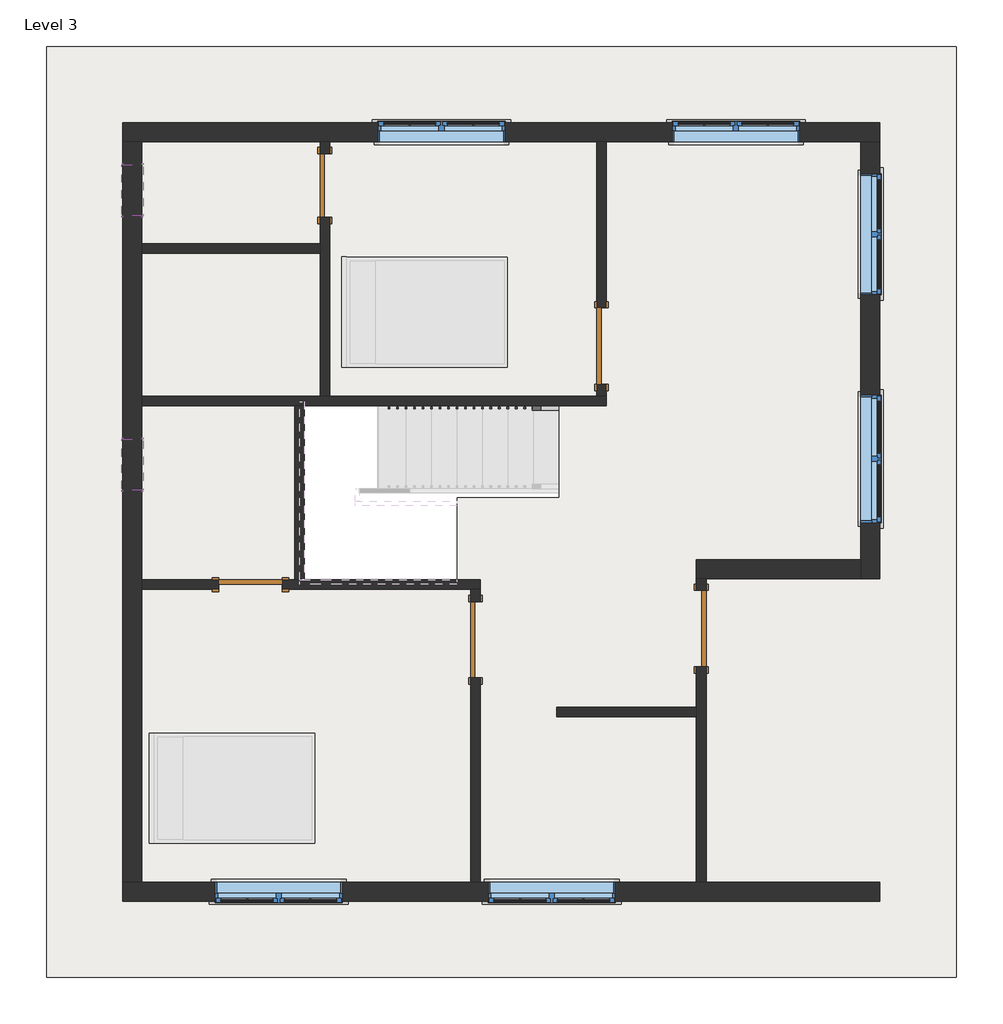
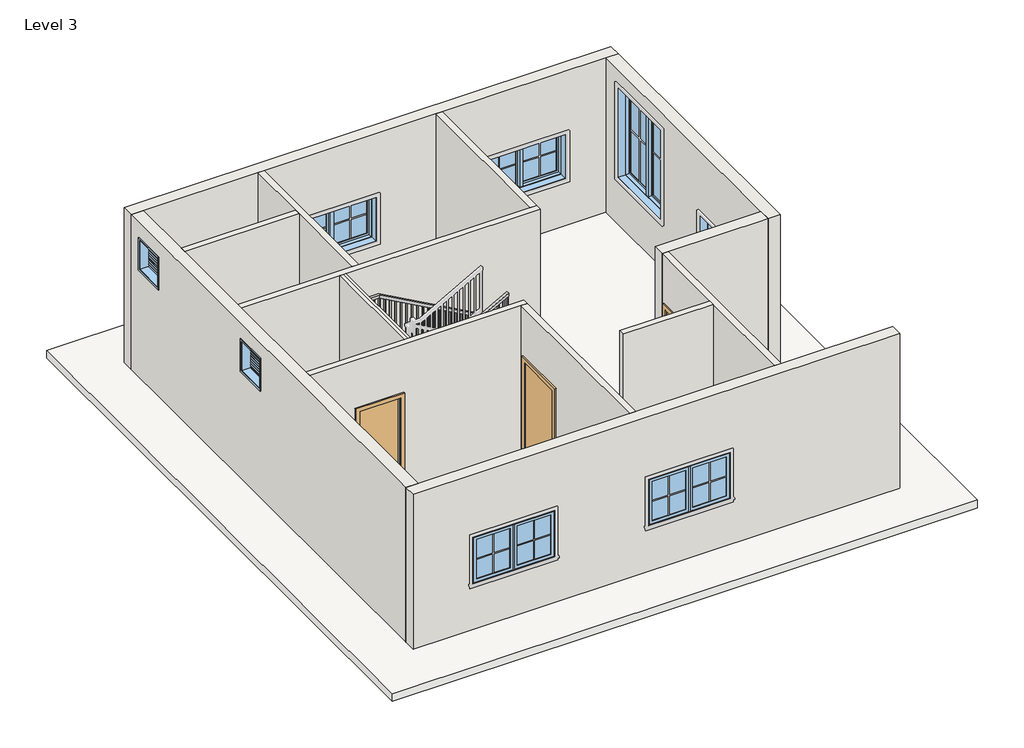
# One storey, part 1 of 2: 14 walls, 8 windows, 5 doors, 1 railing, 1 roof.
"""IFC4 building model written with IfcOpenShell, lengths in millimetres."""

from ifc_helpers import new_model, si_unit, frame, origin, place, context, project, spatial, polyline, outline, extrude, faceted_brep, transform, mapped, element, save
from components import single_flush_3_17d80c48, single_flush_3_5e62189b, door_d8f5dbb5, window_9ac97e1a, window_c1d95f0f, window_f2d8fef0

model = new_model("IFC4")

# Units and contexts
model_context = context("Model", 3, world=origin())
ifc_project = project(units=[si_unit("LENGTHUNIT", "METRE", prefix="MILLI")], contexts=[model_context])

# Site, building, storey
site = spatial("IfcSite", under=ifc_project)
building = spatial("IfcBuilding", under=site)
storey = spatial("IfcBuildingStorey", under=building, Name="Level 3", Elevation=6248.4)

# Doors
placement = place(None, origin())
single_flush_3_shape = single_flush_3_17d80c48(model_context)
element("IfcDoor", 1, ObjectType="Single-Flush : 3'", at=placement, inside=storey, context=model_context, shape_type="MappedRepresentation", body=[
    mapped(single_flush_3_shape, transform((-1566.5130704, -2143.0042021, 6248.4), x_axis=(0.0, 1.0, 0.0), y_axis=(-1.0, 0.0, 0.0), z_axis=(0.0, 0.0, 1.0))),
])
single_flush_3_2_shape = single_flush_3_5e62189b(model_context)
element("IfcDoor", 2, ObjectType="Single-Flush : 3'", at=placement, inside=storey, context=model_context, shape_type="MappedRepresentation", body=[
    mapped(single_flush_3_2_shape, transform((1138.5869296, -2009.6542021, 6248.4), x_axis=(0.0, 1.0, 0.0), y_axis=(-1.0, 0.0, 0.0), z_axis=(0.0, 0.0, 1.0))),
])
element("IfcDoor", 3, ObjectType="Single-Flush : 3'", at=placement, inside=storey, context=model_context, shape_type="MappedRepresentation", body=[
    mapped(single_flush_3_2_shape, transform((-55.2130704, 1374.8957979, 6248.4), x_axis=(0.0, -1.0, 0.0), y_axis=(1.0, 0.0, 0.0), z_axis=(0.0, 0.0, 1.0))),
])
door_shape = door_d8f5dbb5(model_context)
element("IfcDoor", 4, ObjectType="Single-Flush : DOOR 2'6\"", at=placement, inside=storey, context=model_context, shape_type="MappedRepresentation", body=[
    mapped(door_shape, transform((-3369.9130704, 3298.9457979, 6248.4), x_axis=(0.0, 1.0, 0.0), y_axis=(-1.0, 0.0, 0.0), z_axis=(0.0, 0.0, 1.0))),
])
element("IfcDoor", 5, ObjectType="Single-Flush : DOOR 2'6\"", at=placement, inside=storey, context=model_context, shape_type="MappedRepresentation", body=[
    mapped(door_shape, transform((-4258.9130704, -1482.6042021, 6248.4), x_axis=(1.0, 0.0, 0.0), y_axis=(0.0, 1.0, 0.0), z_axis=(0.0, 0.0, 1.0))),
])

# Railing
element("IfcRailing", 6, ObjectType="Handrail - Rectangular", at=placement, inside=storey, context=model_context, shape_type="SolidModel", body=[
    faceted_brep([(-569.5630704, 606.5457979, 7332.1333333), (-569.5630704, 606.5457979, 7274.020221), (-569.5630704, 657.3457979, 7274.020221), (-569.5630704, 657.3457979, 7332.1333333), (-3007.9630704, 606.5457979, 8686.8), (-3021.1266727, 606.5457979, 8636.0), (-3021.1266727, 657.3457979, 8636.0), (-3007.9630704, 657.3457979, 8686.8), (-3566.7630704, 606.5457979, 8686.8), (-3566.7630704, 606.5457979, 8636.0), (-3617.5630704, 657.3457979, 8636.0), (-3617.5630704, 657.3457979, 8686.8), (-3566.7630704, -1374.6542021, 8686.8), (-3566.7630704, -1374.6542021, 8636.0), (-3617.5630704, -1425.4542021, 8636.0), (-3617.5630704, -1425.4542021, 8686.8), (-3312.7630704, -1374.6542021, 8686.8), (-3299.5994682, -1374.6542021, 8636.0), (-3299.5994682, -1425.4542021, 8636.0), (-3312.7630704, -1425.4542021, 8686.8), (-1788.7630704, -1374.6542021, 9533.4666667), (-1788.7630704, -1425.4542021, 9533.4666667), (-1788.7630704, -1425.4542021, 9475.3535543), (-1788.7630704, -1374.6542021, 9475.3535543)], [[[0, 1, 2, 3]], [[1, 0, 4, 5]], [[2, 1, 5, 6]], [[3, 2, 6, 7]], [[0, 3, 7, 4]], [[5, 4, 8, 9]], [[6, 5, 9, 10]], [[7, 6, 10, 11]], [[4, 7, 11, 8]], [[9, 8, 12, 13]], [[10, 9, 13, 14]], [[11, 10, 14, 15]], [[8, 11, 15, 12]], [[13, 12, 16, 17]], [[14, 13, 17, 18]], [[15, 14, 18, 19]], [[12, 15, 19, 16]], [[20, 21, 22, 23]], [[17, 16, 20, 23]], [[18, 17, 23, 22]], [[19, 18, 22, 21]], [[16, 19, 21, 20]]]),
    extrude(outline(polyline([(9438.3118876, -1855.4380704), (9427.7285543, -1874.4880704), (8449.7333333, -1874.4880704), (8449.7333333, -1855.4380704), (9438.3118876, -1855.4380704)])), frame((0.0, -1409.5792021, 0.0), z_axis=(0.0, 1.0, 0.0), x_axis=(0.0, 0.0, 1.0)), (0.0, 0.0, 1.0), 19.05),
    extrude(outline(polyline([(9381.8674432, -1957.0380704), (9371.2841099, -1976.0880704), (8449.7333333, -1976.0880704), (8449.7333333, -1957.0380704), (9381.8674432, -1957.0380704)])), frame((0.0, -1409.5792021, 0.0), z_axis=(0.0, 1.0, 0.0), x_axis=(0.0, 0.0, 1.0)), (0.0, 0.0, 1.0), 19.05),
    extrude(outline(polyline([(9325.4229988, -2058.6380704), (9314.8396654, -2077.6880704), (8449.7333333, -2077.6880704), (8449.7333333, -2058.6380704), (9325.4229988, -2058.6380704)])), frame((0.0, -1409.5792021, 0.0), z_axis=(0.0, 1.0, 0.0), x_axis=(0.0, 0.0, 1.0)), (0.0, 0.0, 1.0), 19.05),
    extrude(outline(polyline([(9268.9785543, -2160.2380704), (9258.395221, -2179.2880704), (8280.4, -2179.2880704), (8280.4, -2160.2380704), (9268.9785543, -2160.2380704)])), frame((0.0, -1409.5792021, 0.0), z_axis=(0.0, 1.0, 0.0), x_axis=(0.0, 0.0, 1.0)), (0.0, 0.0, 1.0), 19.05),
    extrude(outline(polyline([(9212.5341099, -2261.8380704), (9201.9507765, -2280.8880704), (8280.4, -2280.8880704), (8280.4, -2261.8380704), (9212.5341099, -2261.8380704)])), frame((0.0, -1409.5792021, 0.0), z_axis=(0.0, 1.0, 0.0), x_axis=(0.0, 0.0, 1.0)), (0.0, 0.0, 1.0), 19.05),
    extrude(outline(polyline([(9156.0896654, -2363.4380704), (9145.5063321, -2382.4880704), (8280.4, -2382.4880704), (8280.4, -2363.4380704), (9156.0896654, -2363.4380704)])), frame((0.0, -1409.5792021, 0.0), z_axis=(0.0, 1.0, 0.0), x_axis=(0.0, 0.0, 1.0)), (0.0, 0.0, 1.0), 19.05),
    extrude(outline(polyline([(9099.645221, -2465.0380704), (9089.0618876, -2484.0880704), (8111.0666667, -2484.0880704), (8111.0666667, -2465.0380704), (9099.645221, -2465.0380704)])), frame((0.0, -1409.5792021, 0.0), z_axis=(0.0, 1.0, 0.0), x_axis=(0.0, 0.0, 1.0)), (0.0, 0.0, 1.0), 19.05),
    extrude(outline(polyline([(9043.2007765, -2566.6380704), (9032.6174432, -2585.6880704), (8111.0666667, -2585.6880704), (8111.0666667, -2566.6380704), (9043.2007765, -2566.6380704)])), frame((0.0, -1409.5792021, 0.0), z_axis=(0.0, 1.0, 0.0), x_axis=(0.0, 0.0, 1.0)), (0.0, 0.0, 1.0), 19.05),
    extrude(outline(polyline([(8986.7563321, -2668.2380704), (8976.1729988, -2687.2880704), (8111.0666667, -2687.2880704), (8111.0666667, -2668.2380704), (8986.7563321, -2668.2380704)])), frame((0.0, -1409.5792021, 0.0), z_axis=(0.0, 1.0, 0.0), x_axis=(0.0, 0.0, 1.0)), (0.0, 0.0, 1.0), 19.05),
    extrude(outline(polyline([(8930.3118876, -2769.8380704), (8919.7285543, -2788.8880704), (7941.7333333, -2788.8880704), (7941.7333333, -2769.8380704), (8930.3118876, -2769.8380704)])), frame((0.0, -1409.5792021, 0.0), z_axis=(0.0, 1.0, 0.0), x_axis=(0.0, 0.0, 1.0)), (0.0, 0.0, 1.0), 19.05),
    extrude(outline(polyline([(8873.8674432, -2871.4380704), (8863.2841099, -2890.4880704), (7941.7333333, -2890.4880704), (7941.7333333, -2871.4380704), (8873.8674432, -2871.4380704)])), frame((0.0, -1409.5792021, 0.0), z_axis=(0.0, 1.0, 0.0), x_axis=(0.0, 0.0, 1.0)), (0.0, 0.0, 1.0), 19.05),
    extrude(outline(polyline([(8817.4229988, -2973.0380704), (8806.8396654, -2992.0880704), (7941.7333333, -2992.0880704), (7941.7333333, -2973.0380704), (8817.4229988, -2973.0380704)])), frame((0.0, -1409.5792021, 0.0), z_axis=(0.0, 1.0, 0.0), x_axis=(0.0, 0.0, 1.0)), (0.0, 0.0, 1.0), 19.05),
    extrude(outline(polyline([(8760.9785543, -3074.6380704), (8750.395221, -3093.6880704), (7772.4, -3093.6880704), (7772.4, -3074.6380704), (8760.9785543, -3074.6380704)])), frame((0.0, -1409.5792021, 0.0), z_axis=(0.0, 1.0, 0.0), x_axis=(0.0, 0.0, 1.0)), (0.0, 0.0, 1.0), 19.05),
    extrude(outline(polyline([(8704.5341099, -3176.2380704), (8693.9507765, -3195.2880704), (7772.4, -3195.2880704), (7772.4, -3176.2380704), (8704.5341099, -3176.2380704)])), frame((0.0, -1409.5792021, 0.0), z_axis=(0.0, 1.0, 0.0), x_axis=(0.0, 0.0, 1.0)), (0.0, 0.0, 1.0), 19.05),
    extrude(outline(polyline([(8648.0896654, -3277.8380704), (8637.5063321, -3296.8880704), (7772.4, -3296.8880704), (7772.4, -3277.8380704), (8648.0896654, -3277.8380704)])), frame((0.0, -1409.5792021, 0.0), z_axis=(0.0, 1.0, 0.0), x_axis=(0.0, 0.0, 1.0)), (0.0, 0.0, 1.0), 19.05),
    extrude(outline(polyline([(-3398.4880704, -1409.5792021), (-3398.4880704, -1390.5292021), (-3379.4380704, -1390.5292021), (-3379.4380704, -1409.5792021), (-3398.4880704, -1409.5792021)])), frame((0.0, 0.0, 7772.4), z_axis=(0.0, 0.0, 1.0), x_axis=(1.0, 0.0, 0.0)), (0.0, 0.0, 1.0), 863.6),
    extrude(outline(polyline([(-3500.0880704, -1409.5792021), (-3500.0880704, -1390.5292021), (-3481.0380704, -1390.5292021), (-3481.0380704, -1409.5792021), (-3500.0880704, -1409.5792021)])), frame((0.0, 0.0, 7772.4), z_axis=(0.0, 0.0, 1.0), x_axis=(1.0, 0.0, 0.0)), (0.0, 0.0, 1.0), 863.6),
    extrude(outline(polyline([(-3601.6880704, -1288.9292021), (-3582.6380704, -1288.9292021), (-3582.6380704, -1307.9792021), (-3601.6880704, -1307.9792021), (-3601.6880704, -1288.9292021)])), frame((0.0, 0.0, 7772.4), z_axis=(0.0, 0.0, 1.0), x_axis=(1.0, 0.0, 0.0)), (0.0, 0.0, 1.0), 863.6),
    extrude(outline(polyline([(-3601.6880704, -1187.3292021), (-3582.6380704, -1187.3292021), (-3582.6380704, -1206.3792021), (-3601.6880704, -1206.3792021), (-3601.6880704, -1187.3292021)])), frame((0.0, 0.0, 7772.4), z_axis=(0.0, 0.0, 1.0), x_axis=(1.0, 0.0, 0.0)), (0.0, 0.0, 1.0), 863.6),
    extrude(outline(polyline([(-3601.6880704, -1085.7292021), (-3582.6380704, -1085.7292021), (-3582.6380704, -1104.7792021), (-3601.6880704, -1104.7792021), (-3601.6880704, -1085.7292021)])), frame((0.0, 0.0, 7772.4), z_axis=(0.0, 0.0, 1.0), x_axis=(1.0, 0.0, 0.0)), (0.0, 0.0, 1.0), 863.6),
    extrude(outline(polyline([(-3601.6880704, -984.1292021), (-3582.6380704, -984.1292021), (-3582.6380704, -1003.1792021), (-3601.6880704, -1003.1792021), (-3601.6880704, -984.1292021)])), frame((0.0, 0.0, 7772.4), z_axis=(0.0, 0.0, 1.0), x_axis=(1.0, 0.0, 0.0)), (0.0, 0.0, 1.0), 863.6),
    extrude(outline(polyline([(-3601.6880704, -882.5292021), (-3582.6380704, -882.5292021), (-3582.6380704, -901.5792021), (-3601.6880704, -901.5792021), (-3601.6880704, -882.5292021)])), frame((0.0, 0.0, 7772.4), z_axis=(0.0, 0.0, 1.0), x_axis=(1.0, 0.0, 0.0)), (0.0, 0.0, 1.0), 863.6),
    extrude(outline(polyline([(-3601.6880704, -780.9292021), (-3582.6380704, -780.9292021), (-3582.6380704, -799.9792021), (-3601.6880704, -799.9792021), (-3601.6880704, -780.9292021)])), frame((0.0, 0.0, 7772.4), z_axis=(0.0, 0.0, 1.0), x_axis=(1.0, 0.0, 0.0)), (0.0, 0.0, 1.0), 863.6),
    extrude(outline(polyline([(-3601.6880704, -679.3292021), (-3582.6380704, -679.3292021), (-3582.6380704, -698.3792021), (-3601.6880704, -698.3792021), (-3601.6880704, -679.3292021)])), frame((0.0, 0.0, 7772.4), z_axis=(0.0, 0.0, 1.0), x_axis=(1.0, 0.0, 0.0)), (0.0, 0.0, 1.0), 863.6),
    extrude(outline(polyline([(-3601.6880704, -577.7292021), (-3582.6380704, -577.7292021), (-3582.6380704, -596.7792021), (-3601.6880704, -596.7792021), (-3601.6880704, -577.7292021)])), frame((0.0, 0.0, 7772.4), z_axis=(0.0, 0.0, 1.0), x_axis=(1.0, 0.0, 0.0)), (0.0, 0.0, 1.0), 863.6),
    extrude(outline(polyline([(-3601.6880704, -476.1292021), (-3582.6380704, -476.1292021), (-3582.6380704, -495.1792021), (-3601.6880704, -495.1792021), (-3601.6880704, -476.1292021)])), frame((0.0, 0.0, 7772.4), z_axis=(0.0, 0.0, 1.0), x_axis=(1.0, 0.0, 0.0)), (0.0, 0.0, 1.0), 863.6),
    extrude(outline(polyline([(-3601.6880704, -374.5292021), (-3582.6380704, -374.5292021), (-3582.6380704, -393.5792021), (-3601.6880704, -393.5792021), (-3601.6880704, -374.5292021)])), frame((0.0, 0.0, 7772.4), z_axis=(0.0, 0.0, 1.0), x_axis=(1.0, 0.0, 0.0)), (0.0, 0.0, 1.0), 863.6),
    extrude(outline(polyline([(-3601.6880704, -272.9292021), (-3582.6380704, -272.9292021), (-3582.6380704, -291.9792021), (-3601.6880704, -291.9792021), (-3601.6880704, -272.9292021)])), frame((0.0, 0.0, 7772.4), z_axis=(0.0, 0.0, 1.0), x_axis=(1.0, 0.0, 0.0)), (0.0, 0.0, 1.0), 863.6),
    extrude(outline(polyline([(-3601.6880704, -171.3292021), (-3582.6380704, -171.3292021), (-3582.6380704, -190.3792021), (-3601.6880704, -190.3792021), (-3601.6880704, -171.3292021)])), frame((0.0, 0.0, 7772.4), z_axis=(0.0, 0.0, 1.0), x_axis=(1.0, 0.0, 0.0)), (0.0, 0.0, 1.0), 863.6),
    extrude(outline(polyline([(-3601.6880704, -69.7292021), (-3582.6380704, -69.7292021), (-3582.6380704, -88.7792021), (-3601.6880704, -88.7792021), (-3601.6880704, -69.7292021)])), frame((0.0, 0.0, 7772.4), z_axis=(0.0, 0.0, 1.0), x_axis=(1.0, 0.0, 0.0)), (0.0, 0.0, 1.0), 863.6),
    extrude(outline(polyline([(-3601.6880704, 31.8707979), (-3582.6380704, 31.8707979), (-3582.6380704, 12.8207979), (-3601.6880704, 12.8207979), (-3601.6880704, 31.8707979)])), frame((0.0, 0.0, 7772.4), z_axis=(0.0, 0.0, 1.0), x_axis=(1.0, 0.0, 0.0)), (0.0, 0.0, 1.0), 863.6),
    extrude(outline(polyline([(-3601.6880704, 133.4707979), (-3582.6380704, 133.4707979), (-3582.6380704, 114.4207979), (-3601.6880704, 114.4207979), (-3601.6880704, 133.4707979)])), frame((0.0, 0.0, 7772.4), z_axis=(0.0, 0.0, 1.0), x_axis=(1.0, 0.0, 0.0)), (0.0, 0.0, 1.0), 863.6),
    extrude(outline(polyline([(-3601.6880704, 235.0707979), (-3582.6380704, 235.0707979), (-3582.6380704, 216.0207979), (-3601.6880704, 216.0207979), (-3601.6880704, 235.0707979)])), frame((0.0, 0.0, 7772.4), z_axis=(0.0, 0.0, 1.0), x_axis=(1.0, 0.0, 0.0)), (0.0, 0.0, 1.0), 863.6),
    extrude(outline(polyline([(-3601.6880704, 336.6707979), (-3582.6380704, 336.6707979), (-3582.6380704, 317.6207979), (-3601.6880704, 317.6207979), (-3601.6880704, 336.6707979)])), frame((0.0, 0.0, 7772.4), z_axis=(0.0, 0.0, 1.0), x_axis=(1.0, 0.0, 0.0)), (0.0, 0.0, 1.0), 863.6),
    extrude(outline(polyline([(-3601.6880704, 438.2707979), (-3582.6380704, 438.2707979), (-3582.6380704, 419.2207979), (-3601.6880704, 419.2207979), (-3601.6880704, 438.2707979)])), frame((0.0, 0.0, 7772.4), z_axis=(0.0, 0.0, 1.0), x_axis=(1.0, 0.0, 0.0)), (0.0, 0.0, 1.0), 863.6),
    extrude(outline(polyline([(-3601.6880704, 539.8707979), (-3582.6380704, 539.8707979), (-3582.6380704, 520.8207979), (-3601.6880704, 520.8207979), (-3601.6880704, 539.8707979)])), frame((0.0, 0.0, 7772.4), z_axis=(0.0, 0.0, 1.0), x_axis=(1.0, 0.0, 0.0)), (0.0, 0.0, 1.0), 863.6),
    extrude(outline(polyline([(-3506.4380704, 641.4707979), (-3506.4380704, 622.4207979), (-3525.4880704, 622.4207979), (-3525.4880704, 641.4707979), (-3506.4380704, 641.4707979)])), frame((0.0, 0.0, 7772.4), z_axis=(0.0, 0.0, 1.0), x_axis=(1.0, 0.0, 0.0)), (0.0, 0.0, 1.0), 863.6),
    extrude(outline(polyline([(-3404.8380704, 641.4707979), (-3404.8380704, 622.4207979), (-3423.8880704, 622.4207979), (-3423.8880704, 641.4707979), (-3404.8380704, 641.4707979)])), frame((0.0, 0.0, 7772.4), z_axis=(0.0, 0.0, 1.0), x_axis=(1.0, 0.0, 0.0)), (0.0, 0.0, 1.0), 863.6),
    extrude(outline(polyline([(-3303.2380704, 641.4707979), (-3303.2380704, 622.4207979), (-3322.2880704, 622.4207979), (-3322.2880704, 641.4707979), (-3303.2380704, 641.4707979)])), frame((0.0, 0.0, 7772.4), z_axis=(0.0, 0.0, 1.0), x_axis=(1.0, 0.0, 0.0)), (0.0, 0.0, 1.0), 863.6),
    extrude(outline(polyline([(-3201.6380704, 641.4707979), (-3201.6380704, 622.4207979), (-3220.6880704, 622.4207979), (-3220.6880704, 641.4707979), (-3201.6380704, 641.4707979)])), frame((0.0, 0.0, 7772.4), z_axis=(0.0, 0.0, 1.0), x_axis=(1.0, 0.0, 0.0)), (0.0, 0.0, 1.0), 863.6),
    extrude(outline(polyline([(-3100.0380704, 641.4707979), (-3100.0380704, 622.4207979), (-3119.0880704, 622.4207979), (-3119.0880704, 641.4707979), (-3100.0380704, 641.4707979)])), frame((0.0, 0.0, 7772.4), z_axis=(0.0, 0.0, 1.0), x_axis=(1.0, 0.0, 0.0)), (0.0, 0.0, 1.0), 863.6),
    extrude(outline(polyline([(8623.395221, -2998.4380704), (8633.9785543, -3017.4880704), (7772.4, -3017.4880704), (7772.4, -2998.4380704), (8623.395221, -2998.4380704)])), frame((0.0, 622.4207979, 0.0), z_axis=(0.0, 1.0, 0.0), x_axis=(0.0, 0.0, 1.0)), (0.0, 0.0, 1.0), 19.05),
    extrude(outline(polyline([(8566.9507765, -2896.8380704), (8577.5341099, -2915.8880704), (7603.0666667, -2915.8880704), (7603.0666667, -2896.8380704), (8566.9507765, -2896.8380704)])), frame((0.0, 622.4207979, 0.0), z_axis=(0.0, 1.0, 0.0), x_axis=(0.0, 0.0, 1.0)), (0.0, 0.0, 1.0), 19.05),
    extrude(outline(polyline([(8510.5063321, -2795.2380704), (8521.0896654, -2814.2880704), (7603.0666667, -2814.2880704), (7603.0666667, -2795.2380704), (8510.5063321, -2795.2380704)])), frame((0.0, 622.4207979, 0.0), z_axis=(0.0, 1.0, 0.0), x_axis=(0.0, 0.0, 1.0)), (0.0, 0.0, 1.0), 19.05),
    extrude(outline(polyline([(8454.0618876, -2693.6380704), (8464.645221, -2712.6880704), (7603.0666667, -2712.6880704), (7603.0666667, -2693.6380704), (8454.0618876, -2693.6380704)])), frame((0.0, 622.4207979, 0.0), z_axis=(0.0, 1.0, 0.0), x_axis=(0.0, 0.0, 1.0)), (0.0, 0.0, 1.0), 19.05),
    extrude(outline(polyline([(8397.6174432, -2592.0380704), (8408.2007765, -2611.0880704), (7433.7333333, -2611.0880704), (7433.7333333, -2592.0380704), (8397.6174432, -2592.0380704)])), frame((0.0, 622.4207979, 0.0), z_axis=(0.0, 1.0, 0.0), x_axis=(0.0, 0.0, 1.0)), (0.0, 0.0, 1.0), 19.05),
    extrude(outline(polyline([(8341.1729988, -2490.4380704), (8351.7563321, -2509.4880704), (7433.7333333, -2509.4880704), (7433.7333333, -2490.4380704), (8341.1729988, -2490.4380704)])), frame((0.0, 622.4207979, 0.0), z_axis=(0.0, 1.0, 0.0), x_axis=(0.0, 0.0, 1.0)), (0.0, 0.0, 1.0), 19.05),
    extrude(outline(polyline([(8284.7285543, -2388.8380704), (8295.3118876, -2407.8880704), (7433.7333333, -2407.8880704), (7433.7333333, -2388.8380704), (8284.7285543, -2388.8380704)])), frame((0.0, 622.4207979, 0.0), z_axis=(0.0, 1.0, 0.0), x_axis=(0.0, 0.0, 1.0)), (0.0, 0.0, 1.0), 19.05),
    extrude(outline(polyline([(8228.2841099, -2287.2380704), (8238.8674432, -2306.2880704), (7264.4, -2306.2880704), (7264.4, -2287.2380704), (8228.2841099, -2287.2380704)])), frame((0.0, 622.4207979, 0.0), z_axis=(0.0, 1.0, 0.0), x_axis=(0.0, 0.0, 1.0)), (0.0, 0.0, 1.0), 19.05),
    extrude(outline(polyline([(8171.8396654, -2185.6380704), (8182.4229988, -2204.6880704), (7264.4, -2204.6880704), (7264.4, -2185.6380704), (8171.8396654, -2185.6380704)])), frame((0.0, 622.4207979, 0.0), z_axis=(0.0, 1.0, 0.0), x_axis=(0.0, 0.0, 1.0)), (0.0, 0.0, 1.0), 19.05),
    extrude(outline(polyline([(8115.395221, -2084.0380704), (8125.9785543, -2103.0880704), (7264.4, -2103.0880704), (7264.4, -2084.0380704), (8115.395221, -2084.0380704)])), frame((0.0, 622.4207979, 0.0), z_axis=(0.0, 1.0, 0.0), x_axis=(0.0, 0.0, 1.0)), (0.0, 0.0, 1.0), 19.05),
    extrude(outline(polyline([(8058.9507765, -1982.4380704), (8069.5341099, -2001.4880704), (7095.0666667, -2001.4880704), (7095.0666667, -1982.4380704), (8058.9507765, -1982.4380704)])), frame((0.0, 622.4207979, 0.0), z_axis=(0.0, 1.0, 0.0), x_axis=(0.0, 0.0, 1.0)), (0.0, 0.0, 1.0), 19.05),
    extrude(outline(polyline([(8002.5063321, -1880.8380704), (8013.0896654, -1899.8880704), (7095.0666667, -1899.8880704), (7095.0666667, -1880.8380704), (8002.5063321, -1880.8380704)])), frame((0.0, 622.4207979, 0.0), z_axis=(0.0, 1.0, 0.0), x_axis=(0.0, 0.0, 1.0)), (0.0, 0.0, 1.0), 19.05),
    extrude(outline(polyline([(7946.0618876, -1779.2380704), (7956.645221, -1798.2880704), (7095.0666667, -1798.2880704), (7095.0666667, -1779.2380704), (7946.0618876, -1779.2380704)])), frame((0.0, 622.4207979, 0.0), z_axis=(0.0, 1.0, 0.0), x_axis=(0.0, 0.0, 1.0)), (0.0, 0.0, 1.0), 19.05),
    extrude(outline(polyline([(7889.6174432, -1677.6380704), (7900.2007765, -1696.6880704), (6925.7333333, -1696.6880704), (6925.7333333, -1677.6380704), (7889.6174432, -1677.6380704)])), frame((0.0, 622.4207979, 0.0), z_axis=(0.0, 1.0, 0.0), x_axis=(0.0, 0.0, 1.0)), (0.0, 0.0, 1.0), 19.05),
    extrude(outline(polyline([(7833.1729988, -1576.0380704), (7843.7563321, -1595.0880704), (6925.7333333, -1595.0880704), (6925.7333333, -1576.0380704), (7833.1729988, -1576.0380704)])), frame((0.0, 622.4207979, 0.0), z_axis=(0.0, 1.0, 0.0), x_axis=(0.0, 0.0, 1.0)), (0.0, 0.0, 1.0), 19.05),
    extrude(outline(polyline([(7776.7285543, -1474.4380704), (7787.3118876, -1493.4880704), (6925.7333333, -1493.4880704), (6925.7333333, -1474.4380704), (7776.7285543, -1474.4380704)])), frame((0.0, 622.4207979, 0.0), z_axis=(0.0, 1.0, 0.0), x_axis=(0.0, 0.0, 1.0)), (0.0, 0.0, 1.0), 19.05),
    extrude(outline(polyline([(7720.2841099, -1372.8380704), (7730.8674432, -1391.8880704), (6756.4, -1391.8880704), (6756.4, -1372.8380704), (7720.2841099, -1372.8380704)])), frame((0.0, 622.4207979, 0.0), z_axis=(0.0, 1.0, 0.0), x_axis=(0.0, 0.0, 1.0)), (0.0, 0.0, 1.0), 19.05),
    extrude(outline(polyline([(7663.8396654, -1271.2380704), (7674.4229988, -1290.2880704), (6756.4, -1290.2880704), (6756.4, -1271.2380704), (7663.8396654, -1271.2380704)])), frame((0.0, 622.4207979, 0.0), z_axis=(0.0, 1.0, 0.0), x_axis=(0.0, 0.0, 1.0)), (0.0, 0.0, 1.0), 19.05),
    extrude(outline(polyline([(7607.395221, -1169.6380704), (7617.9785543, -1188.6880704), (6756.4, -1188.6880704), (6756.4, -1169.6380704), (7607.395221, -1169.6380704)])), frame((0.0, 622.4207979, 0.0), z_axis=(0.0, 1.0, 0.0), x_axis=(0.0, 0.0, 1.0)), (0.0, 0.0, 1.0), 19.05),
    extrude(outline(polyline([(7550.9507765, -1068.0380704), (7561.5341099, -1087.0880704), (6587.0666667, -1087.0880704), (6587.0666667, -1068.0380704), (7550.9507765, -1068.0380704)])), frame((0.0, 622.4207979, 0.0), z_axis=(0.0, 1.0, 0.0), x_axis=(0.0, 0.0, 1.0)), (0.0, 0.0, 1.0), 19.05),
    extrude(outline(polyline([(7494.5063321, -966.4380704), (7505.0896654, -985.4880704), (6587.0666667, -985.4880704), (6587.0666667, -966.4380704), (7494.5063321, -966.4380704)])), frame((0.0, 622.4207979, 0.0), z_axis=(0.0, 1.0, 0.0), x_axis=(0.0, 0.0, 1.0)), (0.0, 0.0, 1.0), 19.05),
    extrude(outline(polyline([(7438.0618876, -864.8380704), (7448.645221, -883.8880704), (6587.0666667, -883.8880704), (6587.0666667, -864.8380704), (7438.0618876, -864.8380704)])), frame((0.0, 622.4207979, 0.0), z_axis=(0.0, 1.0, 0.0), x_axis=(0.0, 0.0, 1.0)), (0.0, 0.0, 1.0), 19.05),
    extrude(outline(polyline([(7381.6174432, -763.2380704), (7392.2007765, -782.2880704), (6417.7333333, -782.2880704), (6417.7333333, -763.2380704), (7381.6174432, -763.2380704)])), frame((0.0, 622.4207979, 0.0), z_axis=(0.0, 1.0, 0.0), x_axis=(0.0, 0.0, 1.0)), (0.0, 0.0, 1.0), 19.05),
    extrude(outline(polyline([(7325.1729988, -661.6380704), (7335.7563321, -680.6880704), (6417.7333333, -680.6880704), (6417.7333333, -661.6380704), (7325.1729988, -661.6380704)])), frame((0.0, 622.4207979, 0.0), z_axis=(0.0, 1.0, 0.0), x_axis=(0.0, 0.0, 1.0)), (0.0, 0.0, 1.0), 19.05),
    extrude(outline(polyline([(-3601.6880704, -1390.5292021), (-3582.6380704, -1390.5292021), (-3582.6380704, -1409.5792021), (-3601.6880704, -1409.5792021), (-3601.6880704, -1390.5292021)])), frame((0.0, 0.0, 7772.4), z_axis=(0.0, 0.0, 1.0), x_axis=(1.0, 0.0, 0.0)), (0.0, 0.0, 1.0), 863.6),
    extrude(outline(polyline([(-3582.6380704, 641.4707979), (-3582.6380704, 622.4207979), (-3601.6880704, 622.4207979), (-3601.6880704, 641.4707979), (-3582.6380704, 641.4707979)])), frame((0.0, 0.0, 7772.4), z_axis=(0.0, 0.0, 1.0), x_axis=(1.0, 0.0, 0.0)), (0.0, 0.0, 1.0), 863.6),
    extrude(outline(polyline([(9475.3535543, -1788.7630704), (9464.770221, -1807.8130704), (8449.7333333, -1807.8130704), (8449.7333333, -1788.7630704), (9475.3535543, -1788.7630704)])), frame((0.0, -1409.5792021, 0.0), z_axis=(0.0, 1.0, 0.0), x_axis=(0.0, 0.0, 1.0)), (0.0, 0.0, 1.0), 19.05),
    extrude(outline(polyline([(7274.020221, -569.5630704), (7284.6035543, -588.6130704), (6417.7333333, -588.6130704), (6417.7333333, -569.5630704), (7274.020221, -569.5630704)])), frame((0.0, 622.4207979, 0.0), z_axis=(0.0, 1.0, 0.0), x_axis=(0.0, 0.0, 1.0)), (0.0, 0.0, 1.0), 19.05),
])

# Roof
element("IfcRoof", 7, ObjectType="roof 6\"", at=placement, inside=storey, context=model_context, shape_type="SweptSolid", body=[
    extrude(outline(polyline([(4192.9369296, 4962.6457979), (4192.9369296, -6187.9542021), (-6703.6630704, -6187.9542021), (-6703.6630704, 4962.6457979), (4192.9369296, 4962.6457979)]), holes=[polyline([(-3668.3630704, 708.1457979), (-3668.3630704, -1476.2542021), (-1788.7630704, -1476.2542021), (-1788.7630704, -434.8542021), (-569.5630704, -434.8542021), (-569.5630704, 708.1457979), (-3668.3630704, 708.1457979)])]), frame((0.0, 0.0, 6096.0), z_axis=(0.0, 0.0, 1.0), x_axis=(1.0, 0.0, 0.0)), (0.0, 0.0, 1.0), 152.4),
])

# Walls
element("IfcWall", 8, ObjectType="WALL 4.5\"", at=placement, inside=storey, context=model_context, shape_type="Brep", body=[
    faceted_brep([(-3427.0630704, 3819.6457979, 6248.4), (-3427.0630704, 3679.9457979, 6248.4), (-3427.0630704, 3679.9457979, 8280.4), (-3427.0630704, 2917.9457979, 8280.4), (-3427.0630704, 2917.9457979, 6248.4), (-3427.0630704, 2600.4457979, 6248.4), (-3427.0630704, 2486.1457979, 6248.4), (-3427.0630704, 771.6457979, 6248.4), (-3427.0630704, 771.6457979, 9296.4), (-3427.0630704, 2486.1457979, 9296.4), (-3427.0630704, 2600.4457979, 9296.4), (-3427.0630704, 3819.6457979, 9296.4), (-3312.7630704, 3679.9457979, 8280.4), (-3312.7630704, 3679.9457979, 6248.4), (-3312.7630704, 3819.6457979, 6248.4), (-3312.7630704, 3819.6457979, 9296.4), (-3312.7630704, 771.6457979, 9296.4), (-3312.7630704, 771.6457979, 6248.4), (-3312.7630704, 2917.9457979, 6248.4), (-3312.7630704, 2917.9457979, 8280.4)], [[[0, 1, 2, 3, 4, 5, 6, 7, 8, 9, 10, 11]], [[12, 13, 14, 15, 16, 17, 18, 19]], [[18, 17, 7, 6, 5, 4]], [[14, 13, 1, 0]], [[0, 11, 15, 14]], [[8, 7, 17, 16]], [[2, 1, 13, 12]], [[3, 2, 12, 19]], [[4, 3, 19, 18]], [[11, 10, 9, 8, 16, 15]]]),
])
element("IfcWall", 9, ObjectType="WALL 4.5\"", at=placement, inside=storey, context=model_context, shape_type="Brep", body=[
    faceted_brep([(-5560.6630704, 657.3457979, 6248.4), (-3731.8630704, 657.3457979, 6248.4), (-3617.5630704, 657.3457979, 6248.4), (1.9369296, 657.3457979, 6248.4), (1.9369296, 657.3457979, 9296.4), (-3617.5630704, 657.3457979, 9296.4), (-3731.8630704, 657.3457979, 9296.4), (-5560.6630704, 657.3457979, 9296.4), (-5560.6630704, 771.6457979, 6248.4), (-5560.6630704, 771.6457979, 9296.4), (-3427.0630704, 771.6457979, 9296.4), (-3312.7630704, 771.6457979, 9296.4), (-112.3630704, 771.6457979, 9296.4), (1.9369296, 771.6457979, 9296.4), (1.9369296, 771.6457979, 6248.4), (-112.3630704, 771.6457979, 6248.4), (-3312.7630704, 771.6457979, 6248.4), (-3427.0630704, 771.6457979, 6248.4)], [[[0, 1, 2, 3, 4, 5, 6, 7]], [[8, 9, 10, 11, 12, 13, 14, 15, 16, 17]], [[3, 2, 1, 0, 8, 17, 16, 15, 14]], [[7, 6, 5, 4, 13, 12, 11, 10, 9]], [[0, 7, 9, 8]], [[4, 3, 14, 13]]]),
])
element("IfcWall", 10, ObjectType="WALL 4.5\"", at=placement, inside=storey, context=model_context, shape_type="SweptSolid", body=[
    extrude(outline(polyline([(917.6957979, 8280.4), (917.6957979, 6248.4), (771.6457979, 6248.4), (771.6457979, 9296.4), (3819.6457979, 9296.4), (3819.6457979, 6248.4), (1832.0957979, 6248.4), (1832.0957979, 8280.4), (917.6957979, 8280.4)])), frame((-112.3630704, 0.0, 0.0), z_axis=(1.0, 0.0, 0.0), x_axis=(0.0, 1.0, 0.0)), (0.0, 0.0, 1.0), 114.3),
])
element("IfcWall", 11, ObjectType="WALL 4.5\"", at=placement, inside=storey, context=model_context, shape_type="SweptSolid", body=[
    extrude(outline(polyline([(-3427.0630704, 2486.1457979), (-5560.6630704, 2486.1457979), (-5560.6630704, 2600.4457979), (-3427.0630704, 2600.4457979), (-3427.0630704, 2486.1457979)])), frame((0.0, 0.0, 6248.4), z_axis=(0.0, 0.0, 1.0), x_axis=(1.0, 0.0, 0.0)), (0.0, 0.0, 1.0), 3048.0),
])
element("IfcWall", 12, ObjectType="WALL 4.5\"", at=placement, inside=storey, context=model_context, shape_type="Brep", body=[
    faceted_brep([(-3877.9130704, -1539.7542021, 8280.4), (-3877.9130704, -1539.7542021, 6248.4), (-1623.6630704, -1539.7542021, 6248.4), (-1509.3630704, -1539.7542021, 6248.4), (-1509.3630704, -1539.7542021, 9296.4), (-1623.6630704, -1539.7542021, 9296.4), (-5560.6630704, -1539.7542021, 9296.4), (-5560.6630704, -1539.7542021, 6248.4), (-4639.9130704, -1539.7542021, 6248.4), (-4639.9130704, -1539.7542021, 8280.4), (-1509.3630704, -1425.4542021, 6248.4), (-3617.5630704, -1425.4542021, 6248.4), (-3731.8630704, -1425.4542021, 6248.4), (-3877.9130704, -1425.4542021, 6248.4), (-3877.9130704, -1425.4542021, 8280.4), (-4639.9130704, -1425.4542021, 8280.4), (-4639.9130704, -1425.4542021, 6248.4), (-5560.6630704, -1425.4542021, 6248.4), (-5560.6630704, -1425.4542021, 9296.4), (-3731.8630704, -1425.4542021, 9296.4), (-3617.5630704, -1425.4542021, 9296.4), (-1509.3630704, -1425.4542021, 9296.4)], [[[0, 1, 2, 3, 4, 5, 6, 7, 8, 9]], [[10, 11, 12, 13, 14, 15, 16, 17, 18, 19, 20, 21]], [[8, 7, 17, 16]], [[3, 2, 1, 13, 12, 11, 10]], [[6, 5, 4, 21, 20, 19, 18]], [[7, 6, 18, 17]], [[4, 3, 10, 21]], [[14, 13, 1, 0]], [[15, 14, 0, 9]], [[16, 15, 9, 8]]]),
])
element("IfcWall", 13, ObjectType="WALL 4.5\"", at=placement, inside=storey, context=model_context, shape_type="SweptSolid", body=[
    extrude(outline(polyline([(-1539.7542021, 6248.4), (-1685.8042021, 6248.4), (-1685.8042021, 8280.4), (-2600.2042021, 8280.4), (-2600.2042021, 6248.4), (-5044.9542021, 6248.4), (-5044.9542021, 9296.4), (-1539.7542021, 9296.4), (-1539.7542021, 6248.4)])), frame((-1623.6630704, 0.0, 0.0), z_axis=(1.0, 0.0, 0.0), x_axis=(0.0, 1.0, 0.0)), (0.0, 0.0, 1.0), 114.3),
])
element("IfcWall", 14, ObjectType="WALL 4.5\"", at=placement, inside=storey, context=model_context, shape_type="Brep", body=[
    faceted_brep([(1195.7369296, -1552.4542021, 8280.4), (1195.7369296, -1552.4542021, 6248.4), (1195.7369296, -1412.7542021, 6248.4), (1195.7369296, -1412.7542021, 9296.4), (1195.7369296, -5044.9542021, 9296.4), (1195.7369296, -5044.9542021, 6248.4), (1195.7369296, -2466.8542021, 6248.4), (1195.7369296, -2466.8542021, 8280.4), (1081.4369296, -1412.7542021, 6248.4), (1081.4369296, -1552.4542021, 6248.4), (1081.4369296, -1552.4542021, 8280.4), (1081.4369296, -2466.8542021, 8280.4), (1081.4369296, -2466.8542021, 6248.4), (1081.4369296, -2948.9967683, 6248.4), (1081.4369296, -3063.2967683, 6248.4), (1081.4369296, -5044.9542021, 6248.4), (1081.4369296, -5044.9542021, 9296.4), (1081.4369296, -3063.2967683, 9296.4), (1081.4369296, -2948.9967683, 9296.4), (1081.4369296, -1412.7542021, 9296.4)], [[[0, 1, 2, 3, 4, 5, 6, 7]], [[8, 9, 10, 11, 12, 13, 14, 15, 16, 17, 18, 19]], [[6, 5, 15, 14, 13, 12]], [[2, 1, 9, 8]], [[3, 2, 8, 19]], [[5, 4, 16, 15]], [[10, 9, 1, 0]], [[11, 10, 0, 7]], [[12, 11, 7, 6]], [[4, 3, 19, 18, 17, 16]]]),
])
element("IfcWall", 15, ObjectType="WALL 4.5\"", at=placement, inside=storey, context=model_context, shape_type="SweptSolid", body=[
    extrude(outline(polyline([(-594.9630704, -2948.9967683), (1081.4369296, -2948.9967683), (1081.4369296, -3063.2967683), (-594.9630704, -3063.2967683), (-594.9630704, -2948.9967683)])), frame((0.0, 0.0, 6248.4), z_axis=(0.0, 0.0, 1.0), x_axis=(1.0, 0.0, 0.0)), (0.0, 0.0, 1.0), 3048.0),
])
element("IfcWall", 16, ObjectType="WALL 4.5\"", at=placement, inside=storey, context=model_context, shape_type="SweptSolid", body=[
    extrude(outline(polyline([(9296.4, -3731.8630704), (6248.4, -3731.8630704), (6248.4, -3617.5630704), (9296.4, -3617.5630704), (9296.4, -3668.3630704), (9296.4, -3731.8630704)])), frame((0.0, -1425.4542021, 0.0), z_axis=(0.0, 1.0, 0.0), x_axis=(0.0, 0.0, 1.0)), (0.0, 0.0, 1.0), 2082.8),
])
element("IfcWall", 17, ObjectType="WALL 9\"", at=placement, inside=storey, context=model_context, shape_type="Brep", body=[
    faceted_brep([(-5789.2630704, 3819.6457979, 6248.4), (-5560.6630704, 3819.6457979, 6248.4), (-3427.0630704, 3819.6457979, 6248.4), (-3312.7630704, 3819.6457979, 6248.4), (-112.3630704, 3819.6457979, 6248.4), (1.9369296, 3819.6457979, 6248.4), (3049.9369296, 3819.6457979, 6248.4), (3278.5369296, 3819.6457979, 6248.4), (3278.5369296, 3819.6457979, 9296.4), (3049.9369296, 3819.6457979, 9296.4), (1.9369296, 3819.6457979, 9296.4), (-112.3630704, 3819.6457979, 9296.4), (-3312.7630704, 3819.6457979, 9296.4), (-3427.0630704, 3819.6457979, 9296.4), (-5560.6630704, 3819.6457979, 9296.4), (-5789.2630704, 3819.6457979, 9296.4), (2316.5119296, 3819.6457979, 8077.2), (2316.5119296, 3819.6457979, 7162.8), (792.5119296, 3819.6457979, 7162.8), (792.5119296, 3819.6457979, 8077.2), (-1210.9130704, 3819.6457979, 8077.2), (-1210.9130704, 3819.6457979, 7162.8), (-2734.9130704, 3819.6457979, 7162.8), (-2734.9130704, 3819.6457979, 8077.2), (-5789.2630704, 4048.2457979, 6248.4), (-5789.2630704, 4048.2457979, 9296.4), (3278.5369296, 4048.2457979, 9296.4), (3278.5369296, 4048.2457979, 6248.4), (2316.5119296, 4048.2457979, 8077.2), (792.5119296, 4048.2457979, 8077.2), (792.5119296, 4048.2457979, 7162.8), (2316.5119296, 4048.2457979, 7162.8), (-1210.9130704, 4048.2457979, 8077.2), (-2734.9130704, 4048.2457979, 8077.2), (-2734.9130704, 4048.2457979, 7162.8), (-1210.9130704, 4048.2457979, 7162.8)], [[[0, 1, 2, 3, 4, 5, 6, 7, 8, 9, 10, 11, 12, 13, 14, 15], [16, 17, 18, 19], [20, 21, 22, 23]], [[24, 25, 26, 27], [28, 29, 30, 31], [32, 33, 34, 35]], [[7, 6, 5, 4, 3, 2, 1, 0, 24, 27]], [[8, 7, 27, 26]], [[0, 15, 25, 24]], [[17, 16, 28, 31]], [[18, 17, 31, 30]], [[19, 18, 30, 29]], [[16, 19, 29, 28]], [[21, 20, 32, 35]], [[22, 21, 35, 34]], [[23, 22, 34, 33]], [[20, 23, 33, 32]], [[15, 14, 13, 12, 11, 10, 9, 8, 26, 25]]]),
])
element("IfcWall", 18, ObjectType="WALL 9\"", at=placement, inside=storey, context=model_context, shape_type="Brep", body=[
    faceted_brep([(3049.9369296, 3819.6457979, 6248.4), (3049.9369296, -1184.1542021, 6248.4), (3049.9369296, -1412.7542021, 6248.4), (3049.9369296, -1412.7542021, 9296.4), (3049.9369296, -1184.1542021, 9296.4), (3049.9369296, 3819.6457979, 9296.4), (3049.9369296, -739.6542021, 8077.2), (3049.9369296, -739.6542021, 7162.8), (3049.9369296, 784.3457979, 7162.8), (3049.9369296, 784.3457979, 8077.2), (3049.9369296, 1990.8457979, 8991.6), (3049.9369296, 1990.8457979, 7162.8), (3049.9369296, 3438.6457979, 7162.8), (3049.9369296, 3438.6457979, 8991.6), (3278.5369296, 3819.6457979, 6248.4), (3278.5369296, 3819.6457979, 9296.4), (3278.5369296, -1412.7542021, 9296.4), (3278.5369296, -1412.7542021, 6248.4), (3278.5369296, -739.6542021, 8077.2), (3278.5369296, 784.3457979, 8077.2), (3278.5369296, 784.3457979, 7162.8), (3278.5369296, -739.6542021, 7162.8), (3278.5369296, 1990.8457979, 8991.6), (3278.5369296, 3438.6457979, 8991.6), (3278.5369296, 3438.6457979, 7162.8), (3278.5369296, 1990.8457979, 7162.8)], [[[0, 1, 2, 3, 4, 5], [6, 7, 8, 9], [10, 11, 12, 13]], [[14, 15, 16, 17], [18, 19, 20, 21], [22, 23, 24, 25]], [[2, 1, 0, 14, 17]], [[0, 5, 15, 14]], [[3, 2, 17, 16]], [[7, 6, 18, 21]], [[8, 7, 21, 20]], [[9, 8, 20, 19]], [[6, 9, 19, 18]], [[11, 10, 22, 25]], [[12, 11, 25, 24]], [[13, 12, 24, 23]], [[10, 13, 23, 22]], [[5, 4, 3, 16, 15]]]),
])
element("IfcWall", 19, ObjectType="WALL 9\"", at=placement, inside=storey, context=model_context, shape_type="Brep", body=[
    faceted_brep([(3049.9369296, -1184.1542021, 6248.4), (1081.4369296, -1184.1542021, 6248.4), (1081.4369296, -1184.1542021, 9296.4), (3049.9369296, -1184.1542021, 9296.4), (3049.9369296, -1412.7542021, 6248.4), (3049.9369296, -1412.7542021, 9296.4), (1195.7369296, -1412.7542021, 9296.4), (1081.4369296, -1412.7542021, 9296.4), (1081.4369296, -1412.7542021, 6248.4), (1195.7369296, -1412.7542021, 6248.4)], [[[0, 1, 2, 3]], [[4, 5, 6, 7, 8, 9]], [[1, 0, 4, 9, 8]], [[0, 3, 5, 4]], [[2, 1, 8, 7]], [[3, 2, 7, 6, 5]]]),
])
element("IfcWall", 20, ObjectType="WALL 9\"", at=placement, inside=storey, context=model_context, shape_type="Brep", body=[
    faceted_brep([(3278.5369296, -5044.9542021, 6248.4), (1195.7369296, -5044.9542021, 6248.4), (1081.4369296, -5044.9542021, 6248.4), (-1509.3630704, -5044.9542021, 6248.4), (-1623.6630704, -5044.9542021, 6248.4), (-5560.6630704, -5044.9542021, 6248.4), (-5789.2630704, -5044.9542021, 6248.4), (-5789.2630704, -5044.9542021, 9296.4), (-5560.6630704, -5044.9542021, 9296.4), (-1623.6630704, -5044.9542021, 9296.4), (-1509.3630704, -5044.9542021, 9296.4), (1081.4369296, -5044.9542021, 9296.4), (1195.7369296, -5044.9542021, 9296.4), (3278.5369296, -5044.9542021, 9296.4), (-4684.3630704, -5044.9542021, 8077.2), (-4684.3630704, -5044.9542021, 7162.8), (-3160.3630704, -5044.9542021, 7162.8), (-3160.3630704, -5044.9542021, 8077.2), (-1414.1130704, -5044.9542021, 8077.2), (-1414.1130704, -5044.9542021, 7162.8), (109.8869296, -5044.9542021, 7162.8), (109.8869296, -5044.9542021, 8077.2), (3278.5369296, -5273.5542021, 6248.4), (3278.5369296, -5273.5542021, 9296.4), (-5789.2630704, -5273.5542021, 9296.4), (-5789.2630704, -5273.5542021, 6248.4), (-4684.3630704, -5273.5542021, 8077.2), (-3160.3630704, -5273.5542021, 8077.2), (-3160.3630704, -5273.5542021, 7162.8), (-4684.3630704, -5273.5542021, 7162.8), (-1414.1130704, -5273.5542021, 8077.2), (109.8869296, -5273.5542021, 8077.2), (109.8869296, -5273.5542021, 7162.8), (-1414.1130704, -5273.5542021, 7162.8)], [[[0, 1, 2, 3, 4, 5, 6, 7, 8, 9, 10, 11, 12, 13], [14, 15, 16, 17], [18, 19, 20, 21]], [[22, 23, 24, 25], [26, 27, 28, 29], [30, 31, 32, 33]], [[6, 5, 4, 3, 2, 1, 0, 22, 25]], [[0, 13, 23, 22]], [[7, 6, 25, 24]], [[15, 14, 26, 29]], [[16, 15, 29, 28]], [[17, 16, 28, 27]], [[14, 17, 27, 26]], [[19, 18, 30, 33]], [[20, 19, 33, 32]], [[21, 20, 32, 31]], [[18, 21, 31, 30]], [[13, 12, 11, 10, 9, 8, 7, 24, 23]]]),
])
element("IfcWall", 21, ObjectType="WALL 9\"", at=placement, inside=storey, context=model_context, shape_type="Brep", body=[
    faceted_brep([(-5560.6630704, -5044.9542021, 6248.4), (-5560.6630704, -1539.7542021, 6248.4), (-5560.6630704, -1425.4542021, 6248.4), (-5560.6630704, 657.3457979, 6248.4), (-5560.6630704, 771.6457979, 6248.4), (-5560.6630704, 2486.1457979, 6248.4), (-5560.6630704, 2600.4457979, 6248.4), (-5560.6630704, 3819.6457979, 6248.4), (-5560.6630704, 3819.6457979, 9296.4), (-5560.6630704, 2600.4457979, 9296.4), (-5560.6630704, 2486.1457979, 9296.4), (-5560.6630704, 771.6457979, 9296.4), (-5560.6630704, 657.3457979, 9296.4), (-5560.6630704, -1425.4542021, 9296.4), (-5560.6630704, -1539.7542021, 9296.4), (-5560.6630704, -5044.9542021, 9296.4), (-5560.6630704, 257.2957979, 8991.6), (-5560.6630704, 257.2957979, 8382.0), (-5560.6630704, -352.3042021, 8382.0), (-5560.6630704, -352.3042021, 8991.6), (-5560.6630704, 3543.4207979, 8991.6), (-5560.6630704, 3543.4207979, 8382.0), (-5560.6630704, 2933.8207979, 8382.0), (-5560.6630704, 2933.8207979, 8991.6), (-5789.2630704, -5044.9542021, 6248.4), (-5789.2630704, -5044.9542021, 9296.4), (-5789.2630704, 3819.6457979, 9296.4), (-5789.2630704, 3819.6457979, 6248.4), (-5789.2630704, 257.2957979, 8991.6), (-5789.2630704, -352.3042021, 8991.6), (-5789.2630704, -352.3042021, 8382.0), (-5789.2630704, 257.2957979, 8382.0), (-5789.2630704, 3543.4207979, 8991.6), (-5789.2630704, 2933.8207979, 8991.6), (-5789.2630704, 2933.8207979, 8382.0), (-5789.2630704, 3543.4207979, 8382.0)], [[[0, 1, 2, 3, 4, 5, 6, 7, 8, 9, 10, 11, 12, 13, 14, 15], [16, 17, 18, 19], [20, 21, 22, 23]], [[24, 25, 26, 27], [28, 29, 30, 31], [32, 33, 34, 35]], [[7, 6, 5, 4, 3, 2, 1, 0, 24, 27]], [[0, 15, 25, 24]], [[8, 7, 27, 26]], [[17, 16, 28, 31]], [[18, 17, 31, 30]], [[19, 18, 30, 29]], [[16, 19, 29, 28]], [[21, 20, 32, 35]], [[22, 21, 35, 34]], [[23, 22, 34, 33]], [[20, 23, 33, 32]], [[15, 14, 13, 12, 11, 10, 9, 8, 26, 25]]]),
])

# Windows
window_shape = window_9ac97e1a(model_context)
element("IfcWindow", 22, ObjectType="Window-Casement-Double : 57\" x 72\"", at=placement, inside=storey, context=model_context, shape_type="MappedRepresentation", body=[
    mapped(window_shape, transform((3164.2369296, 2714.7457979, 6248.4), x_axis=(0.0, -1.0, 0.0), y_axis=(1.0, 0.0, 0.0), z_axis=(0.0, 0.0, 1.0))),
])
window_2_shape = window_c1d95f0f(model_context)
element("IfcWindow", 23, ObjectType="Window-Casement-Double : WINDOW 6\"", at=placement, inside=storey, context=model_context, shape_type="MappedRepresentation", body=[
    mapped(window_2_shape, transform((-3922.3630704, -5159.2542021, 6248.4), x_axis=(-1.0, 0.0, 0.0), y_axis=(0.0, -1.0, 0.0), z_axis=(0.0, 0.0, 1.0))),
])
element("IfcWindow", 24, ObjectType="Window-Casement-Double : WINDOW 6\"", at=placement, inside=storey, context=model_context, shape_type="MappedRepresentation", body=[
    mapped(window_2_shape, transform((-652.1130704, -5159.2542021, 6248.4), x_axis=(-1.0, 0.0, 0.0), y_axis=(0.0, -1.0, 0.0), z_axis=(0.0, 0.0, 1.0))),
])
element("IfcWindow", 25, ObjectType="Window-Casement-Double : WINDOW 6\"", at=placement, inside=storey, context=model_context, shape_type="MappedRepresentation", body=[
    mapped(window_2_shape, transform((3164.2369296, 22.3457979, 6248.4), x_axis=(0.0, -1.0, 0.0), y_axis=(1.0, 0.0, 0.0), z_axis=(0.0, 0.0, 1.0))),
])
element("IfcWindow", 26, ObjectType="Window-Casement-Double : WINDOW 6\"", at=placement, inside=storey, context=model_context, shape_type="MappedRepresentation", body=[
    mapped(window_2_shape, transform((1554.5119296, 3933.9457979, 6248.4), x_axis=(1.0, 0.0, 0.0), y_axis=(0.0, 1.0, 0.0), z_axis=(0.0, 0.0, 1.0))),
])
element("IfcWindow", 27, ObjectType="Window-Casement-Double : WINDOW 6\"", at=placement, inside=storey, context=model_context, shape_type="MappedRepresentation", body=[
    mapped(window_2_shape, transform((-1972.9130704, 3933.9457979, 6248.4), x_axis=(1.0, 0.0, 0.0), y_axis=(0.0, 1.0, 0.0), z_axis=(0.0, 0.0, 1.0))),
])
window_3_shape = window_f2d8fef0(model_context)
element("IfcWindow", 28, ObjectType="Window-Louvers : 24\" x 24\"", at=placement, inside=storey, context=model_context, shape_type="MappedRepresentation", body=[
    mapped(window_3_shape, transform((-5668.6130704, -47.5042021, 7467.6), x_axis=(0.0, -1.0, 0.0), y_axis=(1.0, 0.0, 0.0), z_axis=(0.0, 0.0, 1.0))),
])
element("IfcWindow", 29, ObjectType="Window-Louvers : 24\" x 24\"", at=placement, inside=storey, context=model_context, shape_type="MappedRepresentation", body=[
    mapped(window_3_shape, transform((-5668.6130704, 3238.6207979, 7467.6), x_axis=(0.0, -1.0, 0.0), y_axis=(1.0, 0.0, 0.0), z_axis=(0.0, 0.0, 1.0))),
])

save(model, "model.ifc")

# Revit data of these elements
# Type "Single-Flush : 3'"
#   Type Mark = "8"
#   Construction Type Id = "MDOOR"
#   Assembly Code = "C1020"
#   Analytic Construction = "Metal"
#   Thickness = 0' - 2"
#   Heat Transfer Coefficient (U) = 0.651978 BTU/(h·ft²·°F)
#   Height = 6' - 8"
#   Trim Projection Ext = 0' - 1"
#   Trim Projection Int = 0' - 1"
#   Trim Width = 0' - 3"
#   Width = 3' - 0"
#   Define Thermal Properties by = 1
#   Door Material = Door - Panel
#   Frame Material = Door - Frame
#   Visual Light Transmittance = 0
#   Solar Heat Gain Coefficient = 0
#   Function = (empty or 0)
#   Wall Closure = (empty or 0)
# Type "Single-Flush : DOOR 2'6\""
#   Type Mark = "9"
#   Construction Type Id = "MDOOR"
#   Assembly Code = "C1020"
#   Analytic Construction = "Metal"
#   Thickness = 0' - 2"
#   Heat Transfer Coefficient (U) = 0.651978 BTU/(h·ft²·°F)
#   Height = 6' - 8"
#   Trim Projection Ext = 0' - 1"
#   Trim Projection Int = 0' - 1"
#   Trim Width = 0' - 3"
#   Width = 2' - 6"
#   Define Thermal Properties by = 1
#   Door Material = Door - Panel
#   Frame Material = Door - Frame
#   Visual Light Transmittance = 0
#   Solar Heat Gain Coefficient = 0
#   Function = (empty or 0)
#   Wall Closure = (empty or 0)
# Type "Handrail - Rectangular"
#   Assembly Code = "C2010400"
#   built-in parameter 1008612 = 0.0416667 (stored number, unit not read)
#   built-in parameter 1008611 = 0.0416667 (stored number, unit not read)
#   built-in parameter 1008609 = 0.333333 (stored number, unit not read)
#   built-in parameter 1008604 = 0.166667 (stored number, unit not read)
#   built-in parameter 1008603 = 0.166667 (stored number, unit not read)
#   Railing Height = 3' - 0"
#   built-in parameter 1008630 = 2
#   built-in parameter 1008610 = 2
#   built-in parameter 1008618 = Baluster - Square : 3/4"
# Type "roof 6\""
#   Assembly Code = "B1020"
#   Layers, outside or top first: 0' - 6" no material (function 1)
# Type "WALL 4.5\""
#   Assembly Code = "B2010"
#   Layers, outside or top first: 0' - 4 1/2" no material (function 1)
# Type "WALL 9\""
#   Assembly Code = "B2010"
#   Layers, outside or top first: 0' - 9" no material (function 1)
# Type "Window-Casement-Double : 57\" x 72\""
#   Type Mark = "17"
#   Fire Rating = "0.5h"
#   Assembly Code = "B2020100"
#   Analytic Construction = "Double glazing - domestic"
#   Frame Extension [instance default] = 0' - 0 1/4"
#   Window Inset [instance default] = 0' - 0"
#   Wall Thickness [instance default] = 0' - 6"
#   Interior Wall Closure [instance default] = 0' - 2 1/4"
#   Half Width = 2' - 4 1/2"
#   Visual Light Transmittance = 0.81
#   Thermal Resistance (R) = 1.8146 (h·ft²·°F)/BTU
#   Solar Heat Gain Coefficient = 0.76
#   Rough Width = 4' - 9 1/2"
#   Rough Height = 6' - 0 1/2"
#   Height = 6' - 0"
#   Heat Transfer Coefficient (U) = 0.5511 BTU/(h·ft²·°F)
#   Exterior Wall Closure [instance default] = 0' - 1 1/4"
#   Extension Jamb [instance default] = 0' - 2 1/4"
#   Default Sill Height = 3' - 0"
#   Width = 4' - 9"
#   Define Thermal Properties by = 0
#   Muntin Visibility = yes
#   Interior Trim Visibility [instance default] = yes
#   Exterior Trim Visibility [instance default] = yes
#   Extension Jamb Visibility [instance default] = yes
#   Interior Trim Material = Wood - Stained
#   Muntin Pattern = Muntin Pattern_2x2 : Muntin Pattern_2x2
#   Interior Trim = Trim-Window-Interior-Flat : Picture Frame
#   Interior Frame Material = Wood - Stained
#   Glass Panel Material = Glass
#   Exterior Trim Material = Clad - White
#   Exterior Trim = Trim-Window-Exterior-Flat : with Sill
#   Exterior Frame Material = Clad - White
#   Wall Closure = (empty or 0)
# Type "Window-Casement-Double : WINDOW 6\""
#   Type Mark = "18"
#   Fire Rating = "0.5h"
#   Assembly Code = "B2020100"
#   Analytic Construction = "Double glazing - domestic"
#   Frame Extension [instance default] = 0' - 0 1/4"
#   Window Inset [instance default] = 0' - 0"
#   Wall Thickness [instance default] = 0' - 6"
#   Interior Wall Closure [instance default] = 0' - 2 1/4"
#   Half Width = 2' - 6"
#   Visual Light Transmittance = 0.81
#   Thermal Resistance (R) = 1.8146 (h·ft²·°F)/BTU
#   Solar Heat Gain Coefficient = 0.76
#   Rough Width = 5' - 0 1/2"
#   Rough Height = 3' - 0 1/2"
#   Height = 3' - 0"
#   Heat Transfer Coefficient (U) = 0.5511 BTU/(h·ft²·°F)
#   Exterior Wall Closure [instance default] = 0' - 1 1/4"
#   Extension Jamb [instance default] = 0' - 2 1/4"
#   Default Sill Height = 3' - 0"
#   Width = 5' - 0"
#   Muntin Visibility = yes
#   Interior Trim Visibility [instance default] = yes
#   Exterior Trim Visibility [instance default] = yes
#   Extension Jamb Visibility [instance default] = yes
#   Interior Trim Material = Wood - Stained
#   Muntin Pattern = Muntin Pattern_2x2 : Muntin Pattern_2x2
#   Interior Trim = Trim-Window-Interior-Flat : Picture Frame
#   Interior Frame Material = Wood - Stained
#   Glass Panel Material = Glass
#   Exterior Trim Material = Clad - White
#   Exterior Trim = Trim-Window-Exterior-Flat : with Sill
#   Exterior Frame Material = Clad - White
#   Wall Closure = (empty or 0)
# Type "Window-Louvers : 24\" x 24\""
#   Type Mark = "19"
#   Construction Type Id = "GSP4R"
#   Assembly Code = "B20"
#   Analytic Construction = "1/8 in Pilkington single glazing"
#   Visual Light Transmittance = 0.9
#   Thermal Resistance (R) = 1.53941 (h·ft²·°F)/BTU
#   Solar Heat Gain Coefficient = 0.78
#   Max Height = 1' - 11.74264"
#   Height = 2' - 0"
#   Heat Transfer Coefficient (U) = 0.6496 BTU/(h·ft²·°F)
#   Blade Width [instance default] = 1' - 10 1/2"
#   Blade Vertical Thickness = 0' - 0.35355"
#   Blade Thickness = 0' - 0 1/4"
#   Blade Spacing = 0' - 1 1/2"
#   Blade Height = 0' - 1.85355"
#   Blade Depth = 0' - 3"
#   Blade Angle = 45.00°
#   Default Sill Height = 3' - 0"
#   Trim Projection_Exterior = 0' - 0 1/2"
#   Trim Projection_Interior = 0' - 0 1/2"
#   Trim Width_Exterior = 0' - 1 1/2"
#   Trim Width_Interior = 0' - 1 1/2"
#   Width = 2' - 0"
#   Max Blade Count = 12
#   Define Thermal Properties by = 1
#   Blade Count = 12
#   Frame Material = Birch
#   Louver Material = Birch
#   Trim Exterior Material = Birch
#   Trim Interior Material = Birch
#   Wall Closure = (empty or 0)
# Elements 1, 2, 3 (IfcDoor, "Single-Flush : 3'")
#   Phase Created = New Construction
#   Materials on its faces: "Door - Frame", "Door - Panel"
# Elements 4, 5 (IfcDoor, "Single-Flush : DOOR 2'6\"")
#   Phase Created = New Construction
#   Materials on its faces: "Door - Frame", "Door - Panel"
# Element 6 (IfcRailing, "Handrail - Rectangular")
#   Phase Created = New Construction
# Element 7 (IfcRoof, "roof 6\"")
#   built-in parameter 1001705 = 20.5 (stored number, unit not read)
#   built-in parameter 1001701 = -0.5 (stored number, unit not read)
#   built-in parameter 1001710 = 33615
#   Phase Created = New Construction
#   Materials on its faces: "Wood - Stained", "Clad - White"
# Elements 8, 10, 11, 13 (IfcWall, "WALL 4.5\"")
#   Top Offset = 0' - 0"
#   Base Offset = 0' - 0"
#   Unconnected Height = 10' - 0"
#   wall height = 10' - 0"
#   Phase Created = New Construction
#   Base Constraint = Level 3
#   Materials on its faces: "Default Wall"
# Elements 9, 12, 14, 15, 16 (IfcWall, "WALL 4.5\"")
#   Top Offset = 0' - 0"
#   Base Offset = 0' - 0"
#   Unconnected Height = 10' - 0"
#   wall height = 10' - 0"
#   Phase Created = New Construction
#   Base Constraint = Level 3
#   Materials on its faces: "Default Wall", "Wood - Stained"
# Elements 17, 18, 20, 21 (IfcWall, "WALL 9\"")
#   Top Offset = 0' - 0"
#   Base Offset = 0' - 0"
#   Unconnected Height = 10' - 0"
#   wall height = 10' - 0"
#   Phase Created = New Construction
#   Base Constraint = Level 3
#   Materials on its faces: "Default Wall", "Wood - Stained"
# Element 19 (IfcWall, "WALL 9\"")
#   Top Offset = 0' - 0"
#   Base Offset = 0' - 0"
#   Unconnected Height = 10' - 0"
#   wall height = 10' - 0"
#   Phase Created = New Construction
#   Base Constraint = Level 3
#   Materials on its faces: "Wood - Stained", "Default Wall"
# Element 22 (IfcWindow, "Window-Casement-Double : 57\" x 72\"")
#   Mark = "24"
#   Window Inset = 0' - 0"
#   Interior Wall Closure = 0' - 2 1/4"
#   Frame Extension = 0' - 0 1/4"
#   Exterior Wall Closure = 0' - 1 1/4"
#   Interior Trim Visibility = yes
#   Exterior Trim Visibility = yes
#   Phase Created = New Construction
#   Materials on its faces: "Wood - Stained", "Glass", "Clad - White"
# Element 23 (IfcWindow, "Window-Casement-Double : WINDOW 6\"")
#   Mark = "17"
#   Window Inset = 0' - 0"
